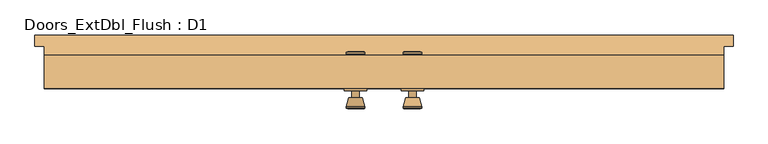
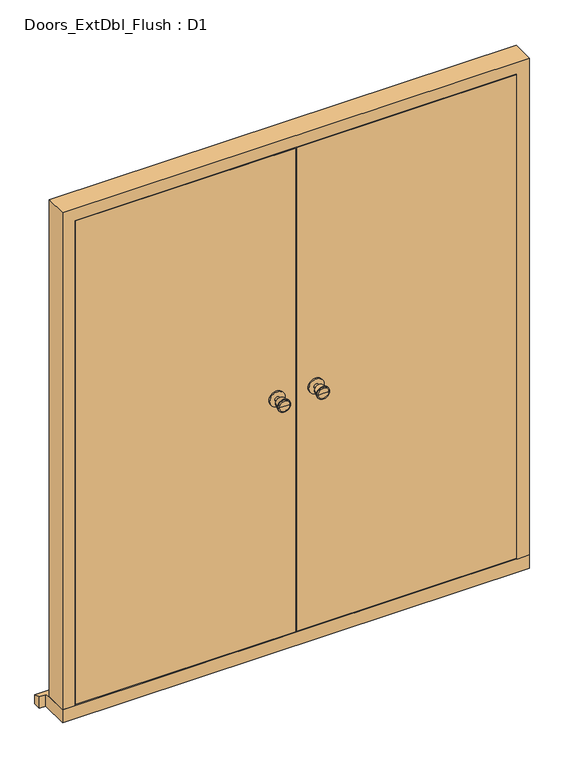
"""IFC4 building model written with IfcOpenShell, lengths in millimetres: door geometry, Doors_ExtDbl_Flush : D1."""

from ifc_helpers import new_model, si_unit, point, frame, frame_2d, origin, place, context, project, spatial, polyline, circle_curve, trimmed, segment, composite_curve, outline, extrude, faceted_brep, source, transform, mapped, element, save
from ifc_brep_helpers import plane_surface, cylinder_surface, revolved_surface, advanced_brep


def doors_extdbl_flush_d1_7bcd4abb(model_context):
    return source(origin(), model_context, "Body", "SolidModel", [
        advanced_brep(
        [(-76.5, -5.7, 1050.0), (-66.5, -5.7, 1050.0), (-86.5, -5.7, 1050.0), (-96.9758676, -54.7, 1050.0), (-56.0241324, -54.7, 1050.0), (-76.5, -54.7, 1050.0), (-101.5, -52.8721319, 1050.0), (-51.5, -52.8721319, 1050.0), (-101.5, -49.4084537, 1050.0), (-51.5, -49.4084537, 1050.0), (-95.136236, -24.7, 1050.0), (-57.863764, -24.7, 1050.0), (-86.5, -24.7, 1050.0), (-66.5, -24.7, 1050.0)],
        [
            (0, 1),
            (1, 2, circle_curve(frame((-76.5, -5.7, 1050.0), z_axis=(0.0, 1.0, 0.0), x_axis=(1.0, 0.0, 0.0)), 10.0)),
            (2, 0),
            (2, 1, circle_curve(frame((-76.5, -5.7, 1050.0), z_axis=(0.0, 1.0, 0.0), x_axis=(1.0, 0.0, 0.0)), 10.0)),
            (3, 4, circle_curve(frame((-76.5, -54.7, 1050.0), z_axis=(0.0, -1.0, 0.0), x_axis=(1.0, 0.0, 0.0)), 20.4758676)),
            (4, 5),
            (5, 3),
            (4, 3, circle_curve(frame((-76.5, -54.7, 1050.0), z_axis=(0.0, -1.0, 0.0), x_axis=(1.0, 0.0, 0.0)), 20.4758676)),
            (6, 7, circle_curve(frame((-76.5, -52.8721319, 1050.0), z_axis=(0.0, -1.0, 0.0), x_axis=(1.0, 0.0, 0.0)), 25.0)),
            (7, 4),
            (3, 6),
            (7, 6, circle_curve(frame((-76.5, -52.8721319, 1050.0), z_axis=(0.0, -1.0, 0.0), x_axis=(1.0, 0.0, 0.0)), 25.0)),
            (8, 9, circle_curve(frame((-76.5, -49.4084537, 1050.0), z_axis=(0.0, -1.0, 0.0), x_axis=(1.0, 0.0, 0.0)), 25.0)),
            (9, 7),
            (6, 8),
            (9, 8, circle_curve(frame((-76.5, -49.4084537, 1050.0), z_axis=(0.0, -1.0, 0.0), x_axis=(1.0, 0.0, 0.0)), 25.0)),
            (10, 11, circle_curve(frame((-76.5, -24.7, 1050.0), z_axis=(0.0, -1.0, 0.0), x_axis=(1.0, 0.0, 0.0)), 18.636236)),
            (11, 9),
            (8, 10),
            (11, 10, circle_curve(frame((-76.5, -24.7, 1050.0), z_axis=(0.0, -1.0, 0.0), x_axis=(1.0, 0.0, 0.0)), 18.636236)),
            (12, 13, circle_curve(frame((-76.5, -24.7, 1050.0), z_axis=(0.0, -1.0, 0.0), x_axis=(1.0, 0.0, 0.0)), 10.0)),
            (13, 11),
            (10, 12),
            (13, 12, circle_curve(frame((-76.5, -24.7, 1050.0), z_axis=(0.0, -1.0, 0.0), x_axis=(1.0, 0.0, 0.0)), 10.0)),
            (1, 13),
            (12, 2),
        ],
        [
            plane_surface(frame((-76.5, -5.7, 1050.0), z_axis=(0.0, 1.0, 0.0), x_axis=(1.0, 0.0, 0.0))),
            plane_surface(frame((-76.5, -54.7, 1050.0), z_axis=(0.0, -1.0, 0.0), x_axis=(1.0, 0.0, 0.0))),
            revolved_surface(polyline([(-56.0241324, -54.7, 1050.0), (-51.5, -52.8721319, 1050.0)]), (-76.5, -5.7, 1050.0), (0.0, 1.0, 0.0)),
            cylinder_surface(frame((-76.5, -5.7, 1050.0), z_axis=(0.0, 1.0, 0.0), x_axis=(1.0, 0.0, 0.0)), 25.0),
            revolved_surface(polyline([(-51.5, -49.4084537, 1050.0), (-57.863764, -24.7, 1050.0)]), (-76.5, -5.7, 1050.0), (0.0, 1.0, 0.0)),
            plane_surface(frame((-76.5, -24.7, 1050.0), z_axis=(0.0, 1.0, 0.0), x_axis=(1.0, 0.0, 0.0))),
            cylinder_surface(frame((-76.5, -5.7, 1050.0), z_axis=(0.0, 1.0, 0.0), x_axis=(1.0, 0.0, 0.0)), 10.0),
        ],
        [
            (0, [[1, 2, 3]]),
            (0, [[-3, 4, -1]]),
            (1, [[5, 6, 7]]),
            (1, [[8, -7, -6]]),
            (2, [[9, 10, -5, 11]]),
            (2, [[12, -11, -8, -10]]),
            (3, [[13, 14, -9, 15]]),
            (3, [[16, -15, -12, -14]]),
            (4, [[17, 18, -13, 19]]),
            (4, [[20, -19, -16, -18]]),
            (5, [[21, 22, -17, 23]]),
            (5, [[24, -23, -20, -22]]),
            (6, [[-2, 25, -21, 26]]),
            (6, [[-4, -26, -24, -25]]),
        ],
    ),
        extrude(outline(composite_curve([segment(trimmed(circle_curve(frame_2d((1050.0, -76.5)), 30.0), [point((1050.0, -46.5))], [point((1050.0, -106.5))], False, "CARTESIAN"), True, "CONTINUOUS"), segment(trimmed(circle_curve(frame_2d((1050.0, -76.5)), 30.0), [point((1050.0, -106.5))], [point((1050.0, -46.5))], False, "CARTESIAN"), True, "CONTINUOUS")], self_intersect=False)), frame((0.0, -5.7, 0.0), z_axis=(0.0, 1.0, 0.0), x_axis=(0.0, 0.0, 1.0)), (0.0, 0.0, 1.0), 6.0),
        advanced_brep(
        [(-76.5, 50.3, 1050.0), (-86.5, 50.3, 1050.0), (-66.5, 50.3, 1050.0), (-96.9758676, 99.3, 1050.0), (-76.5, 99.3, 1050.0), (-56.0241324, 99.3, 1050.0), (-101.5, 97.4721319, 1050.0), (-51.5, 97.4721319, 1050.0), (-101.5, 94.0084537, 1050.0), (-51.5, 94.0084537, 1050.0), (-95.136236, 69.3, 1050.0), (-57.863764, 69.3, 1050.0), (-86.5, 69.3, 1050.0), (-66.5, 69.3, 1050.0)],
        [
            (0, 1),
            (1, 2, circle_curve(frame((-76.5, 50.3, 1050.0), z_axis=(0.0, -1.0, 0.0), x_axis=(1.0, 0.0, 0.0)), 10.0)),
            (2, 0),
            (2, 1, circle_curve(frame((-76.5, 50.3, 1050.0), z_axis=(0.0, -1.0, 0.0), x_axis=(1.0, 0.0, 0.0)), 10.0)),
            (3, 4),
            (4, 5),
            (5, 3, circle_curve(frame((-76.5, 99.3, 1050.0), z_axis=(0.0, 1.0, 0.0), x_axis=(1.0, 0.0, 0.0)), 20.4758676)),
            (3, 5, circle_curve(frame((-76.5, 99.3, 1050.0), z_axis=(0.0, 1.0, 0.0), x_axis=(1.0, 0.0, 0.0)), 20.4758676)),
            (6, 3),
            (5, 7),
            (7, 6, circle_curve(frame((-76.5, 97.4721319, 1050.0), z_axis=(0.0, 1.0, 0.0), x_axis=(1.0, 0.0, 0.0)), 25.0)),
            (6, 7, circle_curve(frame((-76.5, 97.4721319, 1050.0), z_axis=(0.0, 1.0, 0.0), x_axis=(1.0, 0.0, 0.0)), 25.0)),
            (8, 6),
            (7, 9),
            (9, 8, circle_curve(frame((-76.5, 94.0084537, 1050.0), z_axis=(0.0, 1.0, 0.0), x_axis=(1.0, 0.0, 0.0)), 25.0)),
            (8, 9, circle_curve(frame((-76.5, 94.0084537, 1050.0), z_axis=(0.0, 1.0, 0.0), x_axis=(1.0, 0.0, 0.0)), 25.0)),
            (10, 8),
            (9, 11),
            (11, 10, circle_curve(frame((-76.5, 69.3, 1050.0), z_axis=(0.0, 1.0, 0.0), x_axis=(1.0, 0.0, 0.0)), 18.636236)),
            (10, 11, circle_curve(frame((-76.5, 69.3, 1050.0), z_axis=(0.0, 1.0, 0.0), x_axis=(1.0, 0.0, 0.0)), 18.636236)),
            (12, 10),
            (11, 13),
            (13, 12, circle_curve(frame((-76.5, 69.3, 1050.0), z_axis=(0.0, 1.0, 0.0), x_axis=(1.0, 0.0, 0.0)), 10.0)),
            (12, 13, circle_curve(frame((-76.5, 69.3, 1050.0), z_axis=(0.0, 1.0, 0.0), x_axis=(1.0, 0.0, 0.0)), 10.0)),
            (1, 12),
            (13, 2),
        ],
        [
            plane_surface(frame((-76.5, 50.3, 1050.0), z_axis=(0.0, -1.0, 0.0), x_axis=(1.0, 0.0, 0.0))),
            plane_surface(frame((-76.5, 99.3, 1050.0), z_axis=(0.0, 1.0, 0.0), x_axis=(1.0, 0.0, 0.0))),
            revolved_surface(polyline([(-56.0241324, 99.3, 1050.0), (-51.5, 97.4721319, 1050.0)]), (-76.5, 50.3, 1050.0), (0.0, -1.0, 0.0)),
            cylinder_surface(frame((-76.5, 50.3, 1050.0), z_axis=(0.0, -1.0, 0.0), x_axis=(1.0, 0.0, 0.0)), 25.0),
            revolved_surface(polyline([(-51.5, 94.0084537, 1050.0), (-57.863764, 69.3, 1050.0)]), (-76.5, 50.3, 1050.0), (0.0, -1.0, 0.0)),
            plane_surface(frame((-76.5, 69.3, 1050.0), z_axis=(0.0, -1.0, 0.0), x_axis=(1.0, 0.0, 0.0))),
            cylinder_surface(frame((-76.5, 50.3, 1050.0), z_axis=(0.0, -1.0, 0.0), x_axis=(1.0, 0.0, 0.0)), 10.0),
        ],
        [
            (0, [[1, 2, 3]]),
            (0, [[-3, 4, -1]]),
            (1, [[5, 6, 7]]),
            (1, [[-6, -5, 8]]),
            (2, [[9, -7, 10, 11]]),
            (2, [[-10, -8, -9, 12]]),
            (3, [[13, -11, 14, 15]]),
            (3, [[-14, -12, -13, 16]]),
            (4, [[17, -15, 18, 19]]),
            (4, [[-18, -16, -17, 20]]),
            (5, [[21, -19, 22, 23]]),
            (5, [[-22, -20, -21, 24]]),
            (6, [[25, -23, 26, -2]]),
            (6, [[-26, -24, -25, -4]]),
        ],
    ),
        extrude(outline(composite_curve([segment(trimmed(circle_curve(frame_2d((1050.0, -76.5)), 30.0), [point((1050.0, -46.5))], [point((1050.0, -106.5))], False, "CARTESIAN"), True, "CONTINUOUS"), segment(trimmed(circle_curve(frame_2d((1050.0, -76.5)), 30.0), [point((1050.0, -106.5))], [point((1050.0, -46.5))], False, "CARTESIAN"), True, "CONTINUOUS")], self_intersect=False)), frame((0.0, 44.3, 0.0), z_axis=(0.0, 1.0, 0.0), x_axis=(0.0, 0.0, 1.0)), (0.0, 0.0, 1.0), 6.0),
        advanced_brep(
        [(76.5, -5.7, 1050.0), (86.5, -5.7, 1050.0), (66.5, -5.7, 1050.0), (96.9758676, -54.7, 1050.0), (76.5, -54.7, 1050.0), (56.0241324, -54.7, 1050.0), (101.5, -52.8721319, 1050.0), (51.5, -52.8721319, 1050.0), (101.5, -49.4084537, 1050.0), (51.5, -49.4084537, 1050.0), (95.136236, -24.7, 1050.0), (57.863764, -24.7, 1050.0), (86.5, -24.7, 1050.0), (66.5, -24.7, 1050.0)],
        [
            (0, 1),
            (1, 2, circle_curve(frame((76.5, -5.7, 1050.0), z_axis=(0.0, 1.0, 0.0), x_axis=(-1.0, 0.0, 0.0)), 10.0)),
            (2, 0),
            (2, 1, circle_curve(frame((76.5, -5.7, 1050.0), z_axis=(0.0, 1.0, 0.0), x_axis=(-1.0, 0.0, 0.0)), 10.0)),
            (3, 4),
            (4, 5),
            (5, 3, circle_curve(frame((76.5, -54.7, 1050.0), z_axis=(0.0, -1.0, 0.0), x_axis=(-1.0, 0.0, 0.0)), 20.4758676)),
            (3, 5, circle_curve(frame((76.5, -54.7, 1050.0), z_axis=(0.0, -1.0, 0.0), x_axis=(-1.0, 0.0, 0.0)), 20.4758676)),
            (6, 3),
            (5, 7),
            (7, 6, circle_curve(frame((76.5, -52.8721319, 1050.0), z_axis=(0.0, -1.0, 0.0), x_axis=(-1.0, 0.0, 0.0)), 25.0)),
            (6, 7, circle_curve(frame((76.5, -52.8721319, 1050.0), z_axis=(0.0, -1.0, 0.0), x_axis=(-1.0, 0.0, 0.0)), 25.0)),
            (8, 6),
            (7, 9),
            (9, 8, circle_curve(frame((76.5, -49.4084537, 1050.0), z_axis=(0.0, -1.0, 0.0), x_axis=(-1.0, 0.0, 0.0)), 25.0)),
            (8, 9, circle_curve(frame((76.5, -49.4084537, 1050.0), z_axis=(0.0, -1.0, 0.0), x_axis=(-1.0, 0.0, 0.0)), 25.0)),
            (10, 8),
            (9, 11),
            (11, 10, circle_curve(frame((76.5, -24.7, 1050.0), z_axis=(0.0, -1.0, 0.0), x_axis=(-1.0, 0.0, 0.0)), 18.636236)),
            (10, 11, circle_curve(frame((76.5, -24.7, 1050.0), z_axis=(0.0, -1.0, 0.0), x_axis=(-1.0, 0.0, 0.0)), 18.636236)),
            (12, 10),
            (11, 13),
            (13, 12, circle_curve(frame((76.5, -24.7, 1050.0), z_axis=(0.0, -1.0, 0.0), x_axis=(-1.0, 0.0, 0.0)), 10.0)),
            (12, 13, circle_curve(frame((76.5, -24.7, 1050.0), z_axis=(0.0, -1.0, 0.0), x_axis=(-1.0, 0.0, 0.0)), 10.0)),
            (1, 12),
            (13, 2),
        ],
        [
            plane_surface(frame((76.5, -5.7, 1050.0), z_axis=(0.0, 1.0, 0.0), x_axis=(-1.0, 0.0, 0.0))),
            plane_surface(frame((76.5, -54.7, 1050.0), z_axis=(0.0, -1.0, 0.0), x_axis=(-1.0, 0.0, 0.0))),
            revolved_surface(polyline([(56.0241324, -54.7, 1050.0), (51.5, -52.8721319, 1050.0)]), (76.5, -5.7, 1050.0), (0.0, 1.0, 0.0)),
            cylinder_surface(frame((76.5, -5.7, 1050.0), z_axis=(0.0, 1.0, 0.0), x_axis=(-1.0, 0.0, 0.0)), 25.0),
            revolved_surface(polyline([(51.5, -49.4084537, 1050.0), (57.863764, -24.7, 1050.0)]), (76.5, -5.7, 1050.0), (0.0, 1.0, 0.0)),
            plane_surface(frame((76.5, -24.7, 1050.0), z_axis=(0.0, 1.0, 0.0), x_axis=(-1.0, 0.0, 0.0))),
            cylinder_surface(frame((76.5, -5.7, 1050.0), z_axis=(0.0, 1.0, 0.0), x_axis=(-1.0, 0.0, 0.0)), 10.0),
        ],
        [
            (0, [[1, 2, 3]]),
            (0, [[-3, 4, -1]]),
            (1, [[5, 6, 7]]),
            (1, [[-6, -5, 8]]),
            (2, [[9, -7, 10, 11]]),
            (2, [[-10, -8, -9, 12]]),
            (3, [[13, -11, 14, 15]]),
            (3, [[-14, -12, -13, 16]]),
            (4, [[17, -15, 18, 19]]),
            (4, [[-18, -16, -17, 20]]),
            (5, [[21, -19, 22, 23]]),
            (5, [[-22, -20, -21, 24]]),
            (6, [[25, -23, 26, -2]]),
            (6, [[-26, -24, -25, -4]]),
        ],
    ),
        extrude(outline(composite_curve([segment(trimmed(circle_curve(frame_2d((1050.0, 76.5)), 30.0), [point((1050.0, 46.5))], [point((1050.0, 106.5))], False, "CARTESIAN"), True, "CONTINUOUS"), segment(trimmed(circle_curve(frame_2d((1050.0, 76.5)), 30.0), [point((1050.0, 106.5))], [point((1050.0, 46.5))], False, "CARTESIAN"), True, "CONTINUOUS")], self_intersect=False)), frame((0.0, -5.7, 0.0), z_axis=(0.0, 1.0, 0.0), x_axis=(0.0, 0.0, 1.0)), (0.0, 0.0, 1.0), 6.0),
        advanced_brep(
        [(76.5, 50.3, 1050.0), (66.5, 50.3, 1050.0), (86.5, 50.3, 1050.0), (96.9758676, 99.3, 1050.0), (56.0241324, 99.3, 1050.0), (76.5, 99.3, 1050.0), (101.5, 97.4721319, 1050.0), (51.5, 97.4721319, 1050.0), (101.5, 94.0084537, 1050.0), (51.5, 94.0084537, 1050.0), (95.136236, 69.3, 1050.0), (57.863764, 69.3, 1050.0), (86.5, 69.3, 1050.0), (66.5, 69.3, 1050.0)],
        [
            (0, 1),
            (1, 2, circle_curve(frame((76.5, 50.3, 1050.0), z_axis=(0.0, -1.0, 0.0), x_axis=(-1.0, 0.0, 0.0)), 10.0)),
            (2, 0),
            (2, 1, circle_curve(frame((76.5, 50.3, 1050.0), z_axis=(0.0, -1.0, 0.0), x_axis=(-1.0, 0.0, 0.0)), 10.0)),
            (3, 4, circle_curve(frame((76.5, 99.3, 1050.0), z_axis=(0.0, 1.0, 0.0), x_axis=(-1.0, 0.0, 0.0)), 20.4758676)),
            (4, 5),
            (5, 3),
            (4, 3, circle_curve(frame((76.5, 99.3, 1050.0), z_axis=(0.0, 1.0, 0.0), x_axis=(-1.0, 0.0, 0.0)), 20.4758676)),
            (6, 7, circle_curve(frame((76.5, 97.4721319, 1050.0), z_axis=(0.0, 1.0, 0.0), x_axis=(-1.0, 0.0, 0.0)), 25.0)),
            (7, 4),
            (3, 6),
            (7, 6, circle_curve(frame((76.5, 97.4721319, 1050.0), z_axis=(0.0, 1.0, 0.0), x_axis=(-1.0, 0.0, 0.0)), 25.0)),
            (8, 9, circle_curve(frame((76.5, 94.0084537, 1050.0), z_axis=(0.0, 1.0, 0.0), x_axis=(-1.0, 0.0, 0.0)), 25.0)),
            (9, 7),
            (6, 8),
            (9, 8, circle_curve(frame((76.5, 94.0084537, 1050.0), z_axis=(0.0, 1.0, 0.0), x_axis=(-1.0, 0.0, 0.0)), 25.0)),
            (10, 11, circle_curve(frame((76.5, 69.3, 1050.0), z_axis=(0.0, 1.0, 0.0), x_axis=(-1.0, 0.0, 0.0)), 18.636236)),
            (11, 9),
            (8, 10),
            (11, 10, circle_curve(frame((76.5, 69.3, 1050.0), z_axis=(0.0, 1.0, 0.0), x_axis=(-1.0, 0.0, 0.0)), 18.636236)),
            (12, 13, circle_curve(frame((76.5, 69.3, 1050.0), z_axis=(0.0, 1.0, 0.0), x_axis=(-1.0, 0.0, 0.0)), 10.0)),
            (13, 11),
            (10, 12),
            (13, 12, circle_curve(frame((76.5, 69.3, 1050.0), z_axis=(0.0, 1.0, 0.0), x_axis=(-1.0, 0.0, 0.0)), 10.0)),
            (1, 13),
            (12, 2),
        ],
        [
            plane_surface(frame((76.5, 50.3, 1050.0), z_axis=(0.0, -1.0, 0.0), x_axis=(-1.0, 0.0, 0.0))),
            plane_surface(frame((76.5, 99.3, 1050.0), z_axis=(0.0, 1.0, 0.0), x_axis=(-1.0, 0.0, 0.0))),
            revolved_surface(polyline([(56.0241324, 99.3, 1050.0), (51.5, 97.4721319, 1050.0)]), (76.5, 50.3, 1050.0), (0.0, -1.0, 0.0)),
            cylinder_surface(frame((76.5, 50.3, 1050.0), z_axis=(0.0, -1.0, 0.0), x_axis=(-1.0, 0.0, 0.0)), 25.0),
            revolved_surface(polyline([(51.5, 94.0084537, 1050.0), (57.863764, 69.3, 1050.0)]), (76.5, 50.3, 1050.0), (0.0, -1.0, 0.0)),
            plane_surface(frame((76.5, 69.3, 1050.0), z_axis=(0.0, -1.0, 0.0), x_axis=(-1.0, 0.0, 0.0))),
            cylinder_surface(frame((76.5, 50.3, 1050.0), z_axis=(0.0, -1.0, 0.0), x_axis=(-1.0, 0.0, 0.0)), 10.0),
        ],
        [
            (0, [[1, 2, 3]]),
            (0, [[-3, 4, -1]]),
            (1, [[5, 6, 7]]),
            (1, [[8, -7, -6]]),
            (2, [[9, 10, -5, 11]]),
            (2, [[12, -11, -8, -10]]),
            (3, [[13, 14, -9, 15]]),
            (3, [[16, -15, -12, -14]]),
            (4, [[17, 18, -13, 19]]),
            (4, [[20, -19, -16, -18]]),
            (5, [[21, 22, -17, 23]]),
            (5, [[24, -23, -20, -22]]),
            (6, [[-2, 25, -21, 26]]),
            (6, [[-4, -26, -24, -25]]),
        ],
    ),
        extrude(outline(composite_curve([segment(trimmed(circle_curve(frame_2d((1050.0, 76.5)), 30.0), [point((1050.0, 46.5))], [point((1050.0, 106.5))], False, "CARTESIAN"), True, "CONTINUOUS"), segment(trimmed(circle_curve(frame_2d((1050.0, 76.5)), 30.0), [point((1050.0, 106.5))], [point((1050.0, 46.5))], False, "CARTESIAN"), True, "CONTINUOUS")], self_intersect=False)), frame((0.0, 44.3, 0.0), z_axis=(0.0, 1.0, 0.0), x_axis=(0.0, 0.0, 1.0)), (0.0, 0.0, 1.0), 6.0),
        faceted_brep([(843.9, 89.3, 54.5), (914.4, 89.3, 54.5), (914.4, 0.3, 54.5), (865.9, 0.3, 54.5), (865.9, 47.3, 54.5), (843.9, 47.3, 54.5), (843.9, 89.3, 2039.5), (-843.9, 89.3, 2039.5), (-843.9, 89.3, 54.5), (-914.4, 89.3, 54.5), (-914.4, 89.3, 2110.0), (914.4, 89.3, 2110.0), (914.4, 0.3, 2110.0), (-914.4, 0.3, 2110.0), (-914.4, 0.3, 54.5), (-865.9, 0.3, 54.5), (-865.9, 0.3, 2061.5), (865.9, 0.3, 2061.5), (865.9, 47.3, 2061.5), (-865.9, 47.3, 2061.5), (-865.9, 47.3, 54.5), (-843.9, 47.3, 54.5), (-843.9, 47.3, 2039.5), (843.9, 47.3, 2039.5)], [[[0, 1, 2, 3, 4, 5]], [[1, 0, 6, 7, 8, 9, 10, 11]], [[2, 1, 11, 12]], [[3, 2, 12, 13, 14, 15, 16, 17]], [[4, 3, 17, 18]], [[5, 4, 18, 19, 20, 21, 22, 23]], [[0, 5, 23, 6]], [[7, 22, 21, 8]], [[8, 21, 20, 15, 14, 9]], [[13, 10, 9, 14]], [[19, 16, 15, 20]], [[12, 11, 10, 13]], [[18, 17, 16, 19]], [[6, 23, 22, 7]]]),
        faceted_brep([(939.4, 144.3, 0.0), (939.4, 144.3, 38.5947221), (939.4, 114.3, 47.2703282), (939.4, 114.3, 0.0), (-939.4, 144.3, 38.5947221), (-939.4, 144.3, 0.0), (-939.4, 114.3, 0.0), (-939.4, 114.3, 47.2703282), (914.4, 114.3, 0.0), (914.4, 0.3, 0.0), (-914.4, 0.3, 0.0), (-914.4, 114.3, 0.0), (-914.4, 114.3, 47.2703282), (-914.4, 89.3, 54.5), (914.4, 89.3, 54.5), (914.4, 114.3, 47.2703282), (-914.4, 0.3, 54.5), (914.4, 0.3, 54.5)], [[[0, 1, 2, 3]], [[4, 5, 6, 7]], [[5, 0, 3, 8, 9, 10, 11, 6]], [[1, 0, 5, 4]], [[1, 4, 7, 12, 13, 14, 15, 2]], [[13, 16, 17, 14]], [[16, 10, 9, 17]], [[12, 11, 10, 16, 13]], [[11, 12, 7, 6]], [[8, 15, 14, 17, 9]], [[15, 8, 3, 2]]]),
        extrude(outline(polyline([(862.9, 0.3), (1.5, 0.3), (1.5, 44.3), (862.9, 44.3), (862.9, 0.3)])), frame((0.0, 0.0, 58.5), z_axis=(0.0, 0.0, 1.0), x_axis=(1.0, 0.0, 0.0)), (0.0, 0.0, 1.0), 2000.0),
        extrude(outline(polyline([(-1.5, 0.3), (-862.9, 0.3), (-862.9, 44.3), (-1.5, 44.3), (-1.5, 0.3)])), frame((0.0, 0.0, 58.5), z_axis=(0.0, 0.0, 1.0), x_axis=(1.0, 0.0, 0.0)), (0.0, 0.0, 1.0), 2000.0),
    ])


if __name__ == "__main__":
    model = new_model("IFC4")
    model_context = context("Model", 3, world=origin())
    ifc_project = project(units=[si_unit("LENGTHUNIT", "METRE", prefix="MILLI")], contexts=[model_context])
    site = spatial("IfcSite", under=ifc_project)
    building = spatial("IfcBuilding", under=site)
    placement = place(None, origin())
    doors_extdbl_flush_d1_shape = doors_extdbl_flush_d1_7bcd4abb(model_context)
    element("IfcDoor", 1, ObjectType="Doors_ExtDbl_Flush : D1", at=placement, inside=building, context=model_context, shape_type="MappedRepresentation", body=[
        mapped(doors_extdbl_flush_d1_shape, transform((0.0, 0.0, 0.0), x_axis=(1.0, 0.0, 0.0), y_axis=(0.0, 1.0, 0.0), z_axis=(0.0, 0.0, 1.0))),
    ])
    save(model, "model.ifc")

# Revit data of these elements
# Type "Doors_ExtDbl_Flush : D1"
#   Type Mark = "52"
#   Type Comments = "External Double"
#   Operation = "DoubleDoorSingleSwing"
#   Keynote = "L20"
#   Analytic Construction = "Metal"
#   Wrap Layers (Ext) from Ext = 0.336286 ft
#   Wrap Layers (Int) from Ext = 0.582349 ft
#   Thickness = 0.144357 ft
#   Rough Width = 6.0 ft
#   Rough Height = 6.922572 ft
#   O/A Frame Width = 0.209974 ft
#   Heat Transfer Coefficient (U) = 3.7021 W/(m²·K)
#   Handle Z Distance = 3.444882 ft
#   FrameWidth = 0.137795 ft
#   FrameOffset - External = 0.082021 ft
#   FrameDepth = 0.291995 ft
#   Door Panel Width = 2.826115 ft
#   Door Panel Thickness = 0.144357 ft
#   Door Panel Height = 6.56168 ft
#   Cill Thickness = 0.178806 ft
#   Cill Projection = 0.098425 ft
#   Handle X Distance = 0.246063 ft
#   Height = 6.922572 ft
#   Structural Tolerance = 0.021325 ft
#   Tolerance = 0.009843 ft
#   Undercut = 0.013123 ft
#   Width = 6.0 ft
#   Cill Extension = 0.082021 ft
#   Cavity Closer Width = 0.164042 ft
#   Cavity Closer Offset from Ext = 0.336286 ft
#   Cavity Closer Depth = 0.278871 ft
#   Vis - Ironmongery = yes
#   Vis - Cavity Closers = yes
#   Function = 1
#   Material Door = Door - Panel
#   Material Frame = Door - Frame/Mullion
#   Material Ironmongery = Door - Handle
#   Visual Light Transmittance = 0
#   Thermal Resistance (R) = 0
#   Solar Heat Gain Coefficient = 0
#   Wall Closure = (empty or 0)
# Element 1 (IfcDoor, "Doors_ExtDbl_Flush : D1")
#   Materials on its faces: "Door - Handle", "Door - Frame/Mullion", "Door - Panel"
# Materials
#   "Door - Panel": class "Wood", colour RGB 210 159 95, transparency 0, Keynote = "L20", Cost = 0
#   "Door - Frame/Mullion": class "Wood", colour RGB 212 179 113, transparency 0, Keynote = "L20", Cost = 0
#   "Door - Handle": colour RGB 0 0 0, transparency 0, Keynote = "P21", Cost = 0
